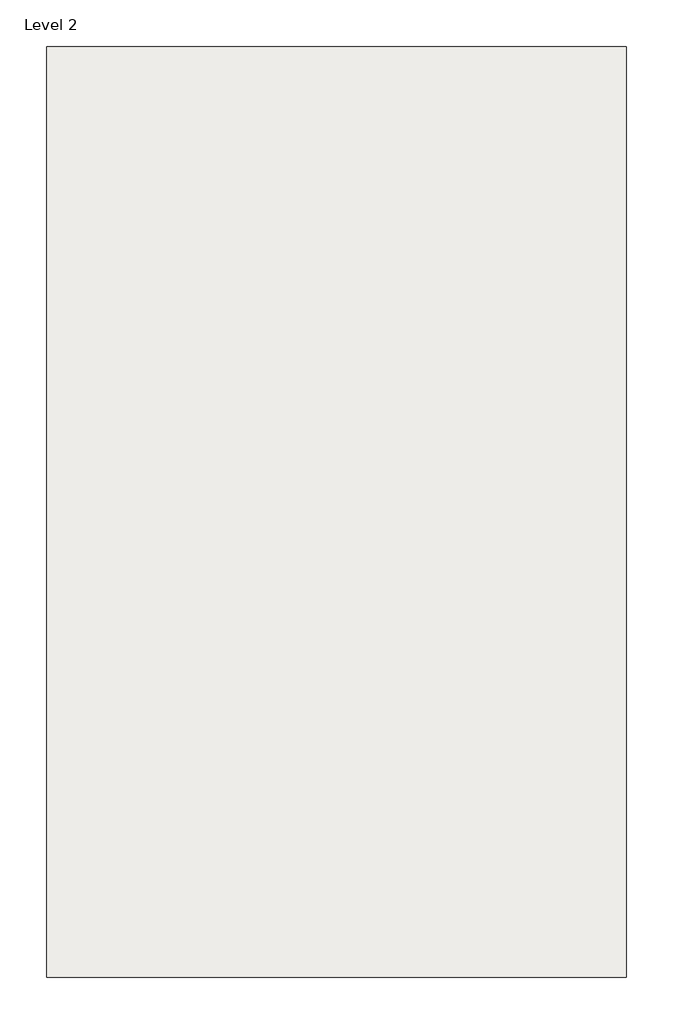
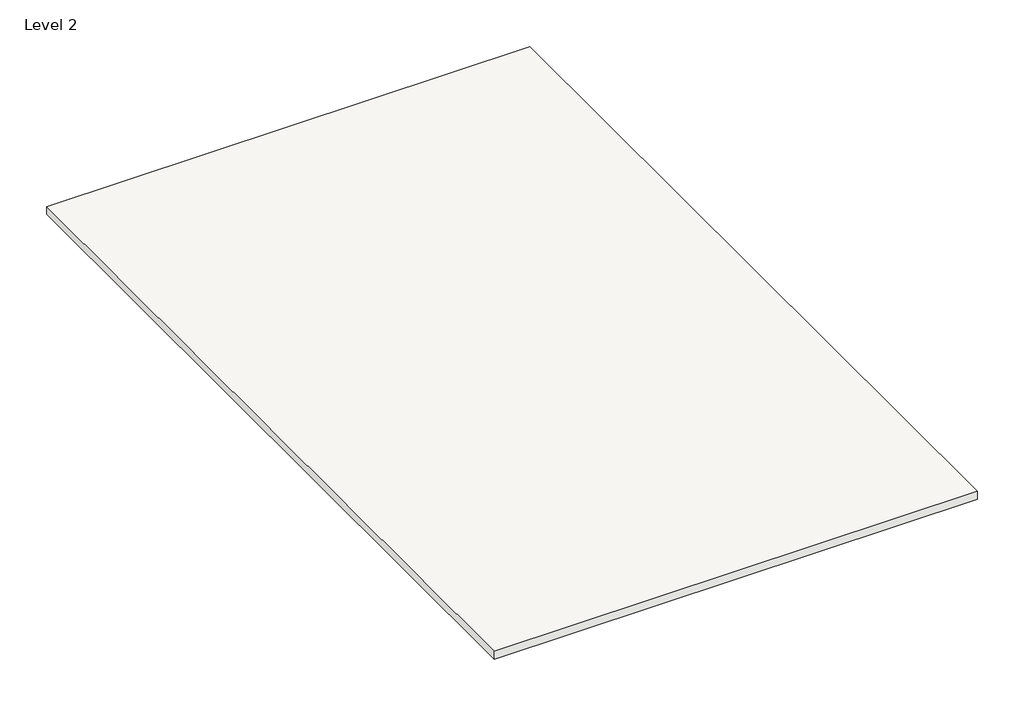
# One storey, incomplete: 1 roof.
"""IFC4 building model written with IfcOpenShell, lengths in millimetres."""

from ifc_helpers import new_model, si_unit, frame, origin, place, context, project, spatial, polyline, outline, extrude, element, save

model = new_model("IFC4")

# Units and contexts
model_context = context("Model", 3, world=origin())
ifc_project = project(units=[si_unit("LENGTHUNIT", "METRE", prefix="MILLI")], contexts=[model_context])

# Site, building, storey
site = spatial("IfcSite", under=ifc_project)
building = spatial("IfcBuilding", under=site)
storey = spatial("IfcBuildingStorey", under=building, Name="Level 2", Elevation=3048.0)

# Roof
placement = place(None, origin())
element("IfcRoof", 1, ObjectType="ROOF 6\"", at=placement, inside=storey, context=model_context, shape_type="SweptSolid", body=[
    extrude(outline(polyline([(-5827.435885, 7397.0649429), (3316.564115, 7397.0649429), (3316.564115, -7284.1350571), (-5827.435885, -7284.1350571), (-5827.435885, 7397.0649429)])), frame((0.0, 0.0, 3048.0), z_axis=(0.0, 0.0, 1.0), x_axis=(1.0, 0.0, 0.0)), (0.0, 0.0, 1.0), 152.4),
])

save(model, "model.ifc")

# Revit data of these elements
# Type "ROOF 6\""
#   Assembly Code = "B1020"
#   Layers, outside or top first: 0' - 6" no material (function 1)
# Element 1 (IfcRoof, "ROOF 6\"")
#   built-in parameter 1001705 = 10.5 (stored number, unit not read)
#   built-in parameter 1001710 = 33615
#   Phase Created = New Construction
#   Materials on its faces: "Default Roof", "Door - Panel"
# Materials
#   "Default Roof": colour RGB 88 101 114, transparency 0, Cost = 0
#   "Door - Panel": class "Wood", colour RGB 210 159 95, transparency 0, Cost = 0
